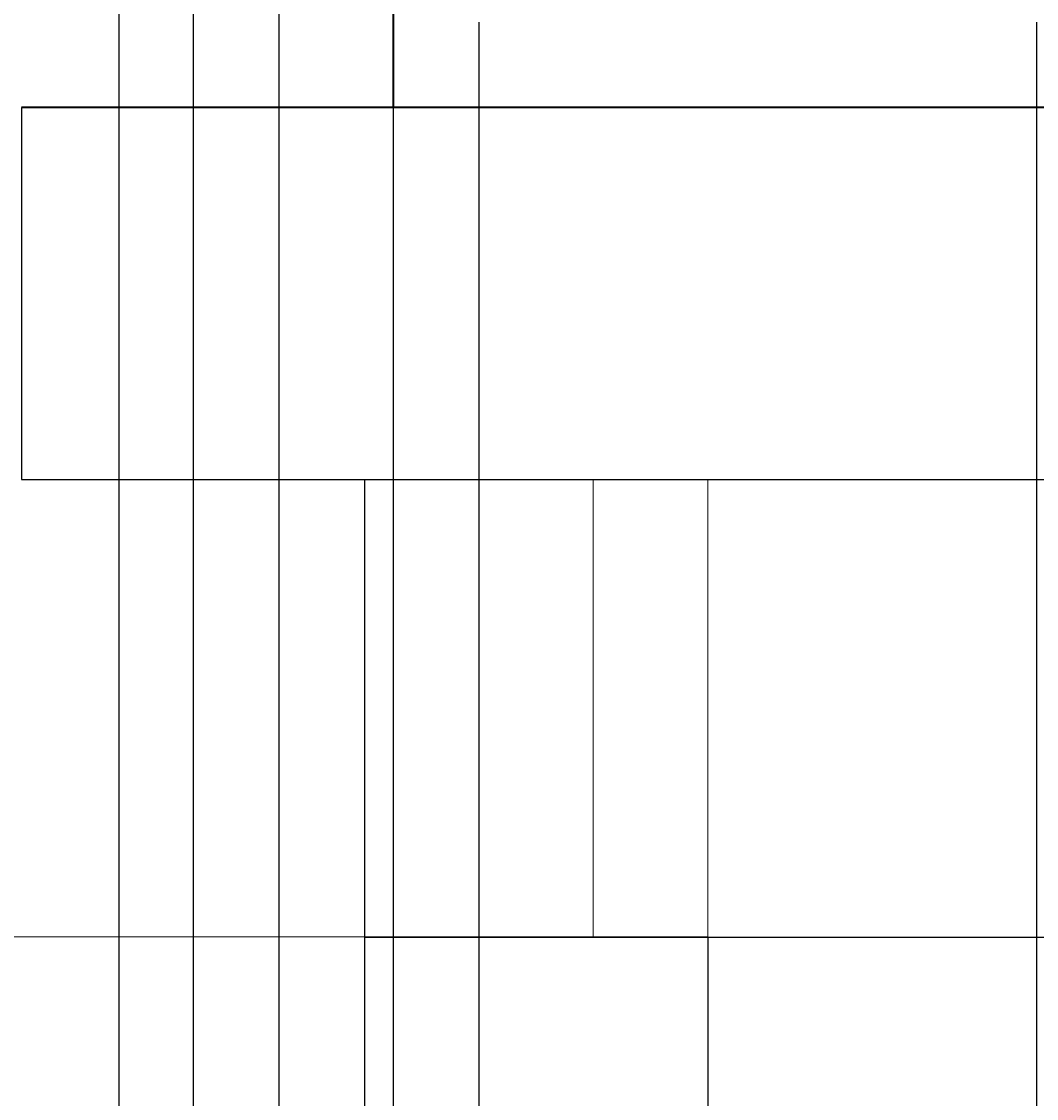
# Model space of a CAD drawing. Units: inches. Extents: x 867 to 1667, y -234 to 788.
# Tile 18 of 42: x 1356 to 1462, y -121 to -8. Entities that reach past the tile are written whole.
import ezdxf

# ---------------------------------------------------------------- set-up
doc = ezdxf.new("R2010")
doc.units = ezdxf.units.IN
doc.header["$MEASUREMENT"] = 0
for name, color, linetype, lineweight in [('A-ANNO-DIMS', 2, 'Continuous', 18), ('A-FLOR-OTLN', 7, 'Continuous', 25), ('A-FLOR-STRS', 7, 'Continuous', 18), ('A-Wall', 7, 'Continuous', 35)]:
    doc.layers.add(name, color=color, linetype=linetype, lineweight=lineweight)
doc.styles.get("Standard").update_dxf_attribs({"font": 'arial.ttf'})
doc.dimstyles.get("Standard").update_dxf_attribs({"dimtxt": 0.6875, "dimasz": 0.18, "dimexe": 0.18, "dimexo": 0.0625, "dimgap": 0.09, "dimtad": 0, "dimdec": 4, "dimzin": 0, "dimdsep": 46, "dimlunit": 4, "dimtxsty": 'Standard', "dimcen": 0.09, "dimadec": 0, "dimazin": 0, "dimtfac": 1, "dimtdec": 4, "dimtofl": 0, "dimtmove": 0, "dimatfit": 3, "dimfxl": 1, "dimtolj": 1, "dimtzin": 0, "dimarcsym": 0})

# ---------------------------------------------------------------- blocks, each defined once
blk = doc.blocks.new('*D23')
at = {"layer": 'A-ANNO-DIMS', "color": 0, "lineweight": -2, "transparency": 16777216}
for p, q in [((1373.89, 623.55), (1373.89, -233.54)), ((1382.89, 623.55), (1382.89, -233.54)), ((1374.07, -233.36), (1378.07, -233.36)), ((1382.71, -233.36), (1378.7, -233.36))]:
    blk.add_line(p, q, dxfattribs=at)
at = {"layer": 'A-ANNO-DIMS', "color": 0, "transparency": 16777216}
for points in [[(1374.07, -233.33), (1374.07, -233.39), (1373.89, -233.36)], [(1382.71, -233.33), (1382.71, -233.39), (1382.89, -233.36)]]:
    blk.add_solid(points, dxfattribs=at)
at = {"layer": 'Defpoints', "color": 0, "transparency": 16777216}
for p in [(1373.89, 623.62), (1382.89, 623.62), (1382.89, -233.36)]:
    blk.add_point(p, dxfattribs=at)
at = {"layer": 'A-ANNO-DIMS', "color": 0, "transparency": 16777216, "insert": (1378.39, -233.36), "char_height": 0.688, "attachment_point": 5}
blk.add_mtext('\\A1;9', dxfattribs=at)
blk = doc.blocks.new('*D27')
at = {"layer": 'A-ANNO-DIMS', "color": 0, "lineweight": -2, "transparency": 16777216}
for p, q in [((1070.89, -55.97), (1070.89, -233.54)), ((1525.26, -186.47), (1525.26, -233.54)), ((1071.07, -233.36), (1296.81, -233.36)), ((1525.08, -233.36), (1299.34, -233.36))]:
    blk.add_line(p, q, dxfattribs=at)
at = {"layer": 'A-ANNO-DIMS', "color": 0, "transparency": 16777216}
for points in [[(1071.07, -233.33), (1071.07, -233.39), (1070.89, -233.36)], [(1525.08, -233.33), (1525.08, -233.39), (1525.26, -233.36)]]:
    blk.add_solid(points, dxfattribs=at)
at = {"layer": 'Defpoints', "color": 0, "transparency": 16777216}
for p in [(1070.89, -55.91), (1525.26, -186.41), (1525.26, -233.36)]:
    blk.add_point(p, dxfattribs=at)
at = {"layer": 'A-ANNO-DIMS', "color": 0, "transparency": 16777216, "insert": (1298.08, -233.36), "char_height": 0.688, "attachment_point": 5}
blk.add_mtext('\\A1;454.4', dxfattribs=at)
blk = doc.blocks.new('*D38')
at = {"layer": 'A-ANNO-DIMS', "color": 0, "lineweight": -2, "transparency": 16777216}
for p, q in [((1403.89, -7.95), (1403.89, -233.54)), ((1559.89, -7.95), (1559.89, -233.54)), ((1404.07, -233.36), (1481.07, -233.36)), ((1559.71, -233.36), (1482.7, -233.36))]:
    blk.add_line(p, q, dxfattribs=at)
at = {"layer": 'A-ANNO-DIMS', "color": 0, "transparency": 16777216}
for points in [[(1404.07, -233.33), (1404.07, -233.39), (1403.89, -233.36)], [(1559.71, -233.33), (1559.71, -233.39), (1559.89, -233.36)]]:
    blk.add_solid(points, dxfattribs=at)
at = {"layer": 'Defpoints', "color": 0, "transparency": 16777216}
for p in [(1403.89, -7.88), (1559.89, -7.88), (1559.89, -233.36)]:
    blk.add_point(p, dxfattribs=at)
at = {"layer": 'A-ANNO-DIMS', "color": 0, "transparency": 16777216, "insert": (1481.89, -233.36), "char_height": 0.688, "attachment_point": 5}
blk.add_mtext('\\A1;156', dxfattribs=at)
blk = doc.blocks.new('*D46')
at = {"layer": 'A-ANNO-DIMS', "color": 0, "lineweight": -2, "transparency": 16777216}
for p, q in [((1256.89, -16.95), (1256.89, -233.54)), ((1394.89, -16.95), (1394.89, -233.54)), ((1257.07, -233.36), (1325.07, -233.36)), ((1394.71, -233.36), (1326.7, -233.36))]:
    blk.add_line(p, q, dxfattribs=at)
at = {"layer": 'A-ANNO-DIMS', "color": 0, "transparency": 16777216}
for points in [[(1257.07, -233.33), (1257.07, -233.39), (1256.89, -233.36)], [(1394.71, -233.33), (1394.71, -233.39), (1394.89, -233.36)]]:
    blk.add_solid(points, dxfattribs=at)
at = {"layer": 'Defpoints', "color": 0, "transparency": 16777216}
for p in [(1256.89, -16.88), (1394.89, -16.88), (1394.89, -233.36)]:
    blk.add_point(p, dxfattribs=at)
at = {"layer": 'A-ANNO-DIMS', "color": 0, "transparency": 16777216, "insert": (1325.89, -233.36), "char_height": 0.688, "attachment_point": 5}
blk.add_mtext('\\A1;138', dxfattribs=at)
blk = doc.blocks.new('*D50')
at = {"layer": 'A-ANNO-DIMS', "color": 0, "lineweight": -2, "transparency": 16777216}
for p, q in [((1211.89, -103.97), (1211.89, -233.54)), ((1427.89, -103.97), (1427.89, -233.54)), ((1212.07, -233.36), (1319.03, -233.36)), ((1427.71, -233.36), (1320.74, -233.36))]:
    blk.add_line(p, q, dxfattribs=at)
at = {"layer": 'A-ANNO-DIMS', "color": 0, "transparency": 16777216}
for points in [[(1212.07, -233.33), (1212.07, -233.39), (1211.89, -233.36)], [(1427.71, -233.33), (1427.71, -233.39), (1427.89, -233.36)]]:
    blk.add_solid(points, dxfattribs=at)
at = {"layer": 'Defpoints', "color": 0, "transparency": 16777216}
for p in [(1211.89, -103.91), (1427.89, -103.91), (1427.89, -233.36)]:
    blk.add_point(p, dxfattribs=at)
at = {"layer": 'A-ANNO-DIMS', "color": 0, "transparency": 16777216, "insert": (1319.89, -233.36), "char_height": 0.688, "attachment_point": 5}
blk.add_mtext('\\A1;216', dxfattribs=at)
blk = doc.blocks.new('*D51')
at = {"layer": 'A-ANNO-DIMS', "color": 0, "lineweight": -2, "transparency": 16777216}
for p, q in [((1391.95, -55.91), (1667.02, -55.91)), ((1666.84, -56.09), (1666.84, -79.31)), ((1666.84, -103.73), (1666.84, -80.51)), ((1391.95, -103.91), (1667.02, -103.91))]:
    blk.add_line(p, q, dxfattribs=at)
at = {"layer": 'A-ANNO-DIMS', "color": 0, "transparency": 16777216}
for points in [[(1666.81, -56.09), (1666.87, -56.09), (1666.84, -55.91)], [(1666.81, -103.73), (1666.87, -103.73), (1666.84, -103.91)]]:
    blk.add_solid(points, dxfattribs=at)
at = {"layer": 'Defpoints', "color": 0, "transparency": 16777216}
for p in [(1391.89, -55.91), (1391.89, -103.91), (1666.84, -103.91)]:
    blk.add_point(p, dxfattribs=at)
at = {"layer": 'A-ANNO-DIMS', "color": 0, "transparency": 16777216, "insert": (1666.84, -79.91), "char_height": 0.688, "attachment_point": 5, "rotation": 90}
blk.add_mtext('\\A1;48', dxfattribs=at)
blk = doc.blocks.new('*D52')
at = {"layer": 'A-ANNO-DIMS', "color": 0, "lineweight": -2, "transparency": 16777216}
for p, q in [((1391.89, -55.97), (1391.89, -233.54)), ((1403.89, -55.97), (1403.89, -233.54)), ((1392.07, -233.36), (1397.34, -233.36)), ((1403.71, -233.36), (1398.43, -233.36))]:
    blk.add_line(p, q, dxfattribs=at)
at = {"layer": 'A-ANNO-DIMS', "color": 0, "transparency": 16777216}
for points in [[(1392.07, -233.33), (1392.07, -233.39), (1391.89, -233.36)], [(1403.71, -233.33), (1403.71, -233.39), (1403.89, -233.36)]]:
    blk.add_solid(points, dxfattribs=at)
at = {"layer": 'Defpoints', "color": 0, "transparency": 16777216}
for p in [(1391.89, -55.91), (1403.89, -55.91), (1403.89, -233.36)]:
    blk.add_point(p, dxfattribs=at)
at = {"layer": 'A-ANNO-DIMS', "color": 0, "transparency": 16777216, "insert": (1397.89, -233.36), "char_height": 0.688, "attachment_point": 5}
blk.add_mtext('\\A1;12', dxfattribs=at)
blk = doc.blocks.new('*D58')
at = {"layer": 'A-ANNO-DIMS', "color": 0, "lineweight": -2, "transparency": 16777216}
for p, q in [((1403.89, -7.95), (1403.89, -233.54)), ((1462.39, -7.95), (1462.39, -233.54)), ((1404.07, -233.36), (1432.15, -233.36)), ((1462.21, -233.36), (1434.12, -233.36))]:
    blk.add_line(p, q, dxfattribs=at)
at = {"layer": 'A-ANNO-DIMS', "color": 0, "transparency": 16777216}
for points in [[(1404.07, -233.33), (1404.07, -233.39), (1403.89, -233.36)], [(1462.21, -233.33), (1462.21, -233.39), (1462.39, -233.36)]]:
    blk.add_solid(points, dxfattribs=at)
at = {"layer": 'Defpoints', "color": 0, "transparency": 16777216}
for p in [(1403.89, -7.88), (1462.39, -7.88), (1462.39, -233.36)]:
    blk.add_point(p, dxfattribs=at)
at = {"layer": 'A-ANNO-DIMS', "color": 0, "transparency": 16777216, "insert": (1433.14, -233.36), "char_height": 0.688, "attachment_point": 5}
blk.add_mtext('\\A1;58.5', dxfattribs=at)
blk = doc.blocks.new('*D60')
at = {"layer": 'A-ANNO-DIMS', "color": 0, "lineweight": -2, "transparency": 16777216}
for p, q in [((1366.11, 136.05), (1366.11, -233.54)), ((1394.89, 136.05), (1394.89, -233.54)), ((1366.29, -233.36), (1379.24, -233.36)), ((1394.71, -233.36), (1381.75, -233.36))]:
    blk.add_line(p, q, dxfattribs=at)
at = {"layer": 'A-ANNO-DIMS', "color": 0, "transparency": 16777216}
for points in [[(1366.29, -233.33), (1366.29, -233.39), (1366.11, -233.36)], [(1394.71, -233.33), (1394.71, -233.39), (1394.89, -233.36)]]:
    blk.add_solid(points, dxfattribs=at)
at = {"layer": 'Defpoints', "color": 0, "transparency": 16777216}
for p in [(1366.11, 136.12), (1394.89, 136.12), (1394.89, -233.36)]:
    blk.add_point(p, dxfattribs=at)
at = {"layer": 'A-ANNO-DIMS', "color": 0, "transparency": 16777216, "insert": (1380.5, -233.36), "char_height": 0.688, "attachment_point": 5}
blk.add_mtext('\\A1;28.78', dxfattribs=at)

msp = doc.modelspace()

# ---------------------------------------------------------------- linework, layer by layer
at = {"layer": 'A-FLOR-OTLN'}
for p, q in [((1355.8866, -16.883), (1355.8866, -55.9081)), ((1355.8866, -55.9081), (1568.8866, -55.9081))]:
    msp.add_line(p, q, dxfattribs=at)
at = {"layer": 'A-FLOR-STRS'}
for p, q in [((1391.8866, -55.9081), (1391.8866, -103.9081)), ((1403.8866, -55.9081), (1403.8866, -103.9081)), ((1415.8866, -55.9081), (1415.8866, -103.9081)), ((1427.8866, -55.9081), (1427.8866, -103.9081)), ((1211.8866, -103.9081), (1427.8866, -103.9081))]:
    msp.add_line(p, q, dxfattribs=at)
at = {"layer": 'A-Wall'}
for p, q in [((1394.8866, 221.617), (1394.8866, -16.883)), ((1568.8866, -16.883), (1355.8866, -16.883))]:
    msp.add_line(p, q, dxfattribs=at)

# ---------------------------------------------------------------- dimensions: what is measured, and where the dimension line sits
at = {"layer": 'A-ANNO-DIMS'}
for base, p1, p2, override, picture, middle in [((1382.8866, -233.3581), (1373.8866, 623.617), (1382.8866, 623.617), {"dimdec": 0, "dimlfac": 1, "dimrnd": 0, "dimzin": 0, "dimdsep": 46, "dimlunit": 2}, '*D23', (1378.3866, -233.3581)), ((1394.8866, -233.3581), (1366.1051, 136.117), (1394.8866, 136.117), {"dimdec": 2, "dimlfac": 1, "dimrnd": 0, "dimzin": 0, "dimdsep": 46, "dimlunit": 2}, '*D60', (1380.4959, -233.3581)), ((1559.8866, -233.3581), (1403.8866, -7.883), (1559.8866, -7.883), {"dimdec": 0, "dimlfac": 1, "dimrnd": 0, "dimzin": 0, "dimdsep": 46, "dimlunit": 2}, '*D38', (1481.8866, -233.3581)), ((1462.3866, -233.3581), (1403.8866, -7.883), (1462.3866, -7.883), {"dimdec": 1, "dimlfac": 1, "dimrnd": 0, "dimzin": 0, "dimdsep": 46, "dimlunit": 2}, '*D58', (1433.1366, -233.3581)), ((1394.8866, -233.3581), (1256.8866, -16.883), (1394.8866, -16.883), {"dimdec": 0, "dimlfac": 1, "dimrnd": 0, "dimzin": 0, "dimdsep": 46, "dimlunit": 2}, '*D46', (1325.8866, -233.3581)), ((1525.2648, -233.3581), (1070.8866, -55.9081), (1525.2648, -186.4081), {"dimdec": 1, "dimlfac": 1, "dimrnd": 0, "dimzin": 0, "dimdsep": 46, "dimlunit": 2}, '*D27', (1298.0757, -233.3581)), ((1403.8866, -233.3581), (1391.8866, -55.9081), (1403.8866, -55.9081), {"dimdec": 0, "dimlfac": 1, "dimrnd": 0, "dimzin": 0, "dimdsep": 46, "dimlunit": 2}, '*D52', (1397.8866, -233.3581)), ((1427.8866, -233.3581), (1211.8866, -103.9081), (1427.8866, -103.9081), {"dimdec": 0, "dimlfac": 1, "dimrnd": 0, "dimzin": 0, "dimdsep": 46, "dimlunit": 2}, '*D50', (1319.8866, -233.3581))]:
    dim = msp.add_linear_dim(base=base, p1=p1, p2=p2, dimstyle='Standard', override=override, dxfattribs=at)
    dim.commit()
    dim.dimension.update_dxf_attribs({"geometry": picture, "text_midpoint": middle})
dim = msp.add_linear_dim(base=(1666.8366, -103.9081), p1=(1391.8866, -55.9081), p2=(1391.8866, -103.9081), angle=90, dimstyle='Standard', override={"dimdec": 0, "dimlfac": 1, "dimrnd": 0, "dimzin": 0, "dimdsep": 46, "dimlunit": 2}, dxfattribs=at)
dim.commit()
dim.dimension.update_dxf_attribs({"geometry": '*D51', "text_midpoint": (1666.8366, -79.9081)})

doc.saveas('drawing.dxf')
